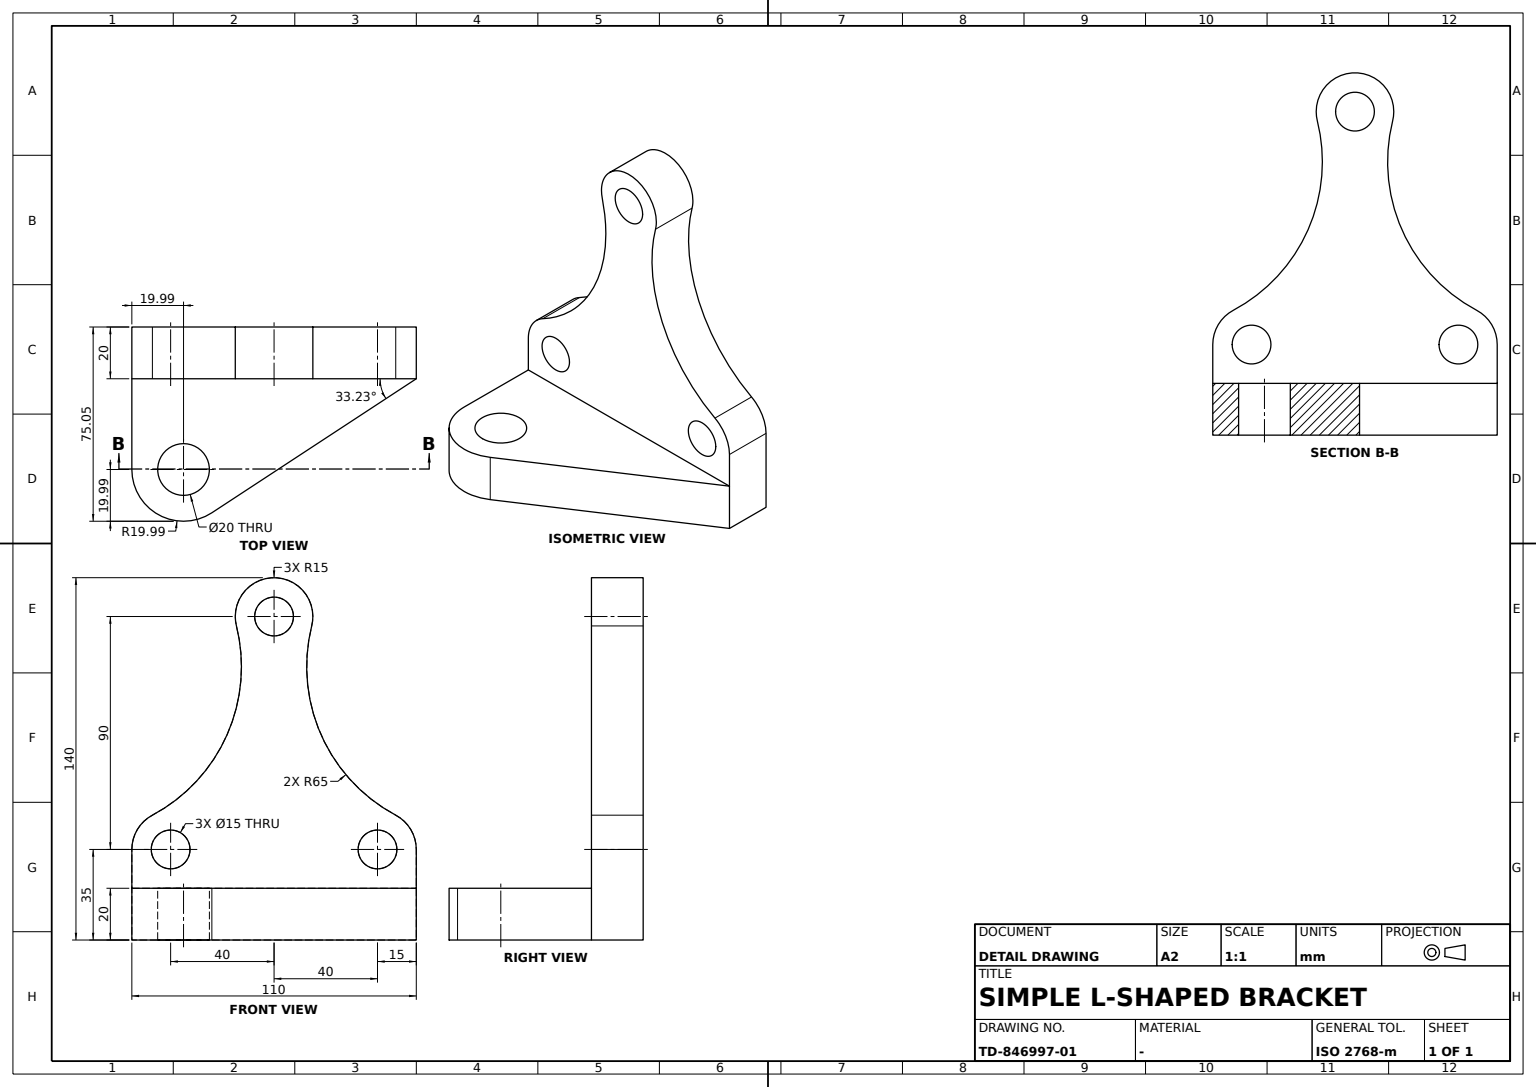
CATIA V5 part; units mm, degrees
sketch "Sketch1" plane through (0, 0, 0) normal (1, 0, 0) x (0, 1, 0)
  circle A0 centre (0, 90) radius 7.5
  point P0 (0, 90)
  circle A1 centre (40, 0) radius 7.5
  point P1 (40, 0)
  circle A2 centre (-40, 0) radius 7.5
  point P2 (-40, 0)
  arc A3 (14.5526, 86.3636) -> (-14.5526, 86.3636) centre (0, 90) ccw
  arc A4 (-47.0526, 13.2386) -> (-55, 0) centre (-40, 0) ccw
  arc A5 (55, 0) -> (47.0526, 13.2386) centre (40, 0) ccw
  arc A6 (-14.5526, 86.3636) -> (-47.0526, 13.2386) centre (-77.6136, 70.6061) cw
  arc A7 (14.5526, 86.3636) -> (47.0526, 13.2386) centre (77.6136, 70.6061) ccw
  line L0 (-55, 0) -> (-55, -35)
  point P3 (-55, 0)
  line L1 (55, 0) -> (55, -35)
  point P4 (55, 0)
  line L2 (-55, -35) -> (55, -35)
  dimension "radius A0" = 7.5
  dimension "distance P0 x axis" = 90
  dimension "radius A1" = 7.5
  dimension "distance P1 y axis" = 40
  dimension "radius A2" = 7.5
  dimension "distance P2 y axis" = 40
  dimension "radius A3" = 15
  dimension "radius A4" = 15
  dimension "radius A5" = 15
  dimension "radius A6" = 65
  dimension "radius A7" = 65
  dimension "length L0" = 35
  constraint coincidence P0 y-axis
  constraint coincidence P1 x-axis
  constraint coincidence P2 x-axis
  constraint coincidence P3 x-axis
  constraint coincidence P4 x-axis
  constraint concentricity A3 A0
  constraint tangency A6 A3
  constraint tangency A6 A4
  constraint tangency A7 A3
  constraint tangency A7 A5
  constraint tangency L0 A4
  constraint tangency L1 A5
  constraint horizontal L2 x-axis
extrude "Pad1" add sketch "Sketch1" along normal blind 20
sketch "Sketch2" plane through (0, 0, -35) normal (0, 0, -1) x (1, 0, 0)
  line L0 (20, 55) -> (55.0611, 55)
  point P0 (20, 55)
  point P1 (60, 55)
  point P2 (20, 55)
  circle A0 centre (55.0611, 35.0088) radius 10
  arc A1 (71.784, 24.0546) -> (55.0611, 55) centre (55.0611, 35.0088) ccw
  point P3 (55.0611, 35.0088)
  line L1 (20, -55) -> (71.784, 24.0546)
  point P4 (20, -55)
  point P5 (20, -55)
  line L2 (20, 55) -> (20, -55) construction
  line L3 (20, 55) -> (20, -55)
  dimension "radius A0" = 10
  dimension "distance P3 L0" = 19.9912
  dimension "distance P3 L2" = 35.0611
  constraint horizontal L0 x-axis
  constraint coincidence P0 P2
  constraint coincidence P4 P5
  constraint tangency A1 L0
  constraint tangency L1 A1
  constraint concentricity A0 A1
  constraint vertical L3 y-axis
extrude "Pad2" add sketch "Sketch2" against normal blind 20
